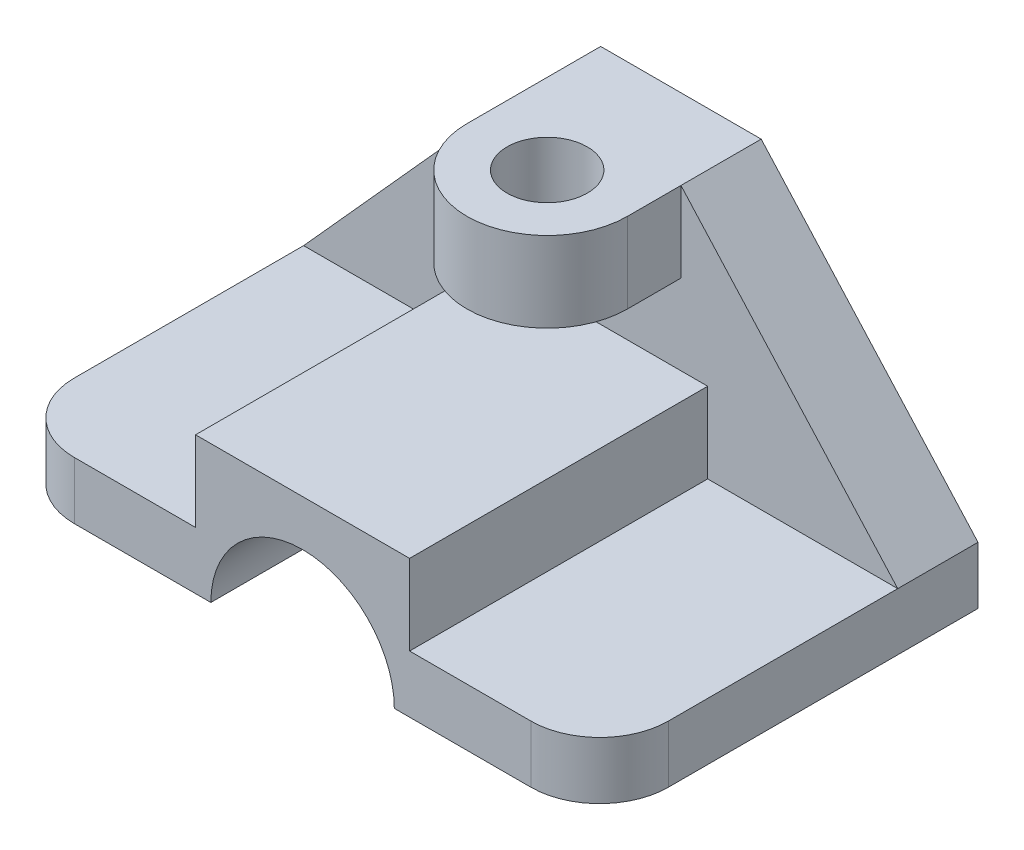
ISO-10303-21;
HEADER;
FILE_DESCRIPTION(('STEP AP214'),'2;1');
FILE_NAME('part.step','',(''),(''),'','','');
FILE_SCHEMA(('AUTOMOTIVE_DESIGN { 1 0 10303 214 1 1 1 1 }'));
ENDSEC;
DATA;
#1=APPLICATION_CONTEXT('core data for automotive mechanical design processes');
#2=APPLICATION_PROTOCOL_DEFINITION('international standard','automotive_design',2000,#1);
#3=PRODUCT_CONTEXT('',#1,'mechanical');
#4=PRODUCT('Part','Part','',(#3));
#5=PRODUCT_RELATED_PRODUCT_CATEGORY('part','',(#4));
#6=PRODUCT_DEFINITION_FORMATION('','',#4);
#7=PRODUCT_DEFINITION_CONTEXT('part definition',#1,'design');
#8=PRODUCT_DEFINITION('design','',#6,#7);
#9=PRODUCT_DEFINITION_SHAPE('','',#8);
#10=(LENGTH_UNIT() NAMED_UNIT(*) SI_UNIT(.MILLI.,.METRE.));
#11=(NAMED_UNIT(*) PLANE_ANGLE_UNIT() SI_UNIT($,.RADIAN.));
#12=(NAMED_UNIT(*) SI_UNIT($,.STERADIAN.) SOLID_ANGLE_UNIT());
#13=UNCERTAINTY_MEASURE_WITH_UNIT(LENGTH_MEASURE(1.E-05),#10,'distance_accuracy_value','');
#14=(GEOMETRIC_REPRESENTATION_CONTEXT(3) GLOBAL_UNCERTAINTY_ASSIGNED_CONTEXT((#13)) GLOBAL_UNIT_ASSIGNED_CONTEXT((#10,
#11,#12)) REPRESENTATION_CONTEXT('',''));
#15=CARTESIAN_POINT('',(0.,0.,0.));
#16=DIRECTION('',(0.,0.,1.));
#17=DIRECTION('',(1.,0.,0.));
#18=AXIS2_PLACEMENT_3D('',#15,#16,#17);
#19=CARTESIAN_POINT('',(-77.7254547907637,-57.,-14.));
#20=DIRECTION('',(0.,-1.,0.));
#21=DIRECTION('',(0.,0.,-1.));
#22=AXIS2_PLACEMENT_3D('',#19,#20,#21);
#23=PLANE('',#22);
#24=DIRECTION('',(0.,0.,1.));
#25=VECTOR('',#24,1.);
#26=CARTESIAN_POINT('',(24.,-57.,-35.001));
#27=LINE('',#26,#25);
#28=CARTESIAN_POINT('',(24.,-57.,-35.));
#29=VERTEX_POINT('',#28);
#30=CARTESIAN_POINT('',(24.,-57.,64.));
#31=VERTEX_POINT('',#30);
#32=EDGE_CURVE('E53',#29,#31,#27,.T.);
#33=ORIENTED_EDGE('',*,*,#32,.F.);
#34=DIRECTION('',(-1.,0.,0.));
#35=VECTOR('',#34,1.);
#36=CARTESIAN_POINT('',(-77.7254547907637,-57.,-35.));
#37=LINE('',#36,#35);
#38=CARTESIAN_POINT('',(77.7254547907637,-57.,-35.));
#39=VERTEX_POINT('',#38);
#40=EDGE_CURVE('E178',#39,#29,#37,.T.);
#41=ORIENTED_EDGE('',*,*,#40,.F.);
#42=DIRECTION('',(0.,0.,-1.));
#43=VECTOR('',#42,1.);
#44=CARTESIAN_POINT('',(77.7254547907637,-57.,-14.));
#45=LINE('',#44,#43);
#46=CARTESIAN_POINT('',(77.7254547907637,-57.,46.));
#47=VERTEX_POINT('',#46);
#48=EDGE_CURVE('E205',#47,#39,#45,.T.);
#49=ORIENTED_EDGE('',*,*,#48,.F.);
#50=CARTESIAN_POINT('',(59.7254547907637,-57.,46.));
#51=DIRECTION('',(0.,-1.,0.));
#52=DIRECTION('',(0.,0.,-1.));
#53=AXIS2_PLACEMENT_3D('',#50,#51,#52);
#54=CIRCLE('',#53,18.);
#55=CARTESIAN_POINT('',(59.7254547907637,-57.,64.));
#56=VERTEX_POINT('',#55);
#57=EDGE_CURVE('E258',#47,#56,#54,.T.);
#58=ORIENTED_EDGE('',*,*,#57,.T.);
#59=DIRECTION('',(1.,0.,0.));
#60=VECTOR('',#59,1.);
#61=CARTESIAN_POINT('',(-77.7254547907637,-57.,64.));
#62=LINE('',#61,#60);
#63=EDGE_CURVE('E263',#31,#56,#62,.T.);
#64=ORIENTED_EDGE('',*,*,#63,.F.);
#65=EDGE_LOOP('',(#33,#41,#49,#58,#64));
#66=FACE_BOUND('',#65,.T.);
#67=ADVANCED_FACE('F39',(#66),#23,.T.);
#68=CARTESIAN_POINT('',(0.,0.,-14.));
#69=DIRECTION('',(0.,0.,1.));
#70=DIRECTION('',(1.,0.,0.));
#71=AXIS2_PLACEMENT_3D('',#68,#69,#70);
#72=PLANE('',#71);
#73=DIRECTION('',(0.,1.,0.));
#74=VECTOR('',#73,1.);
#75=CARTESIAN_POINT('',(28.,-21.,-14.));
#76=LINE('',#75,#74);
#77=CARTESIAN_POINT('',(28.,-42.,-14.));
#78=VERTEX_POINT('',#77);
#79=CARTESIAN_POINT('',(28.,-21.,-14.));
#80=VERTEX_POINT('',#79);
#81=EDGE_CURVE('E294',#78,#80,#76,.T.);
#82=ORIENTED_EDGE('',*,*,#81,.F.);
#83=DIRECTION('',(-1.,0.,0.));
#84=VECTOR('',#83,1.);
#85=CARTESIAN_POINT('',(28.,-42.,-14.));
#86=LINE('',#85,#84);
#87=CARTESIAN_POINT('',(77.7254547907637,-42.,-14.));
#88=VERTEX_POINT('',#87);
#89=EDGE_CURVE('E295',#88,#78,#86,.T.);
#90=ORIENTED_EDGE('',*,*,#89,.F.);
#91=DIRECTION('',(0.669130606358857,-0.743144825477396,0.));
#92=VECTOR('',#91,1.);
#93=CARTESIAN_POINT('',(77.7254547907637,-42.,-14.));
#94=LINE('',#93,#92);
#95=CARTESIAN_POINT('',(21.,21.,-14.));
#96=VERTEX_POINT('',#95);
#97=EDGE_CURVE('E195',#96,#88,#94,.T.);
#98=ORIENTED_EDGE('',*,*,#97,.F.);
#99=DIRECTION('',(0.,1.,0.));
#100=VECTOR('',#99,1.);
#101=CARTESIAN_POINT('',(21.,21.,-14.));
#102=LINE('',#101,#100);
#103=CARTESIAN_POINT('',(21.,0.,-14.));
#104=VERTEX_POINT('',#103);
#105=EDGE_CURVE('E208',#104,#96,#102,.T.);
#106=ORIENTED_EDGE('',*,*,#105,.F.);
#107=DIRECTION('',(1.,0.,0.));
#108=VECTOR('',#107,1.);
#109=CARTESIAN_POINT('',(0.,0.,-14.));
#110=LINE('',#109,#108);
#111=CARTESIAN_POINT('',(-21.,0.,-14.));
#112=VERTEX_POINT('',#111);
#113=EDGE_CURVE('E196',#112,#104,#110,.T.);
#114=ORIENTED_EDGE('',*,*,#113,.F.);
#115=DIRECTION('',(0.,-1.,0.));
#116=VECTOR('',#115,1.);
#117=CARTESIAN_POINT('',(-21.,21.,-14.));
#118=LINE('',#117,#116);
#119=CARTESIAN_POINT('',(-21.,21.,-14.));
#120=VERTEX_POINT('',#119);
#121=EDGE_CURVE('E245',#120,#112,#118,.T.);
#122=ORIENTED_EDGE('',*,*,#121,.F.);
#123=DIRECTION('',(0.669130606358857,0.743144825477396,0.));
#124=VECTOR('',#123,1.);
#125=CARTESIAN_POINT('',(-21.,21.,-14.));
#126=LINE('',#125,#124);
#127=CARTESIAN_POINT('',(-77.7254547907637,-42.,-14.));
#128=VERTEX_POINT('',#127);
#129=EDGE_CURVE('E206',#128,#120,#126,.T.);
#130=ORIENTED_EDGE('',*,*,#129,.F.);
#131=DIRECTION('',(-1.,0.,0.));
#132=VECTOR('',#131,1.);
#133=CARTESIAN_POINT('',(-77.7254547907637,-42.,-14.));
#134=LINE('',#133,#132);
#135=CARTESIAN_POINT('',(-28.,-42.,-14.));
#136=VERTEX_POINT('',#135);
#137=EDGE_CURVE('E297',#136,#128,#134,.T.);
#138=ORIENTED_EDGE('',*,*,#137,.F.);
#139=DIRECTION('',(0.,-1.,0.));
#140=VECTOR('',#139,1.);
#141=CARTESIAN_POINT('',(-28.,-42.,-14.));
#142=LINE('',#141,#140);
#143=CARTESIAN_POINT('',(-28.,-21.,-14.));
#144=VERTEX_POINT('',#143);
#145=EDGE_CURVE('E296',#144,#136,#142,.T.);
#146=ORIENTED_EDGE('',*,*,#145,.F.);
#147=DIRECTION('',(-1.,0.,0.));
#148=VECTOR('',#147,1.);
#149=CARTESIAN_POINT('',(-28.,-21.,-14.));
#150=LINE('',#149,#148);
#151=EDGE_CURVE('E298',#80,#144,#150,.T.);
#152=ORIENTED_EDGE('',*,*,#151,.F.);
#153=EDGE_LOOP('',(#82,#90,#98,#106,#114,#122,#130,#138,#146,#152));
#154=FACE_BOUND('',#153,.T.);
#155=ADVANCED_FACE('F333',(#154),#72,.T.);
#156=CARTESIAN_POINT('',(0.,21.,0.));
#157=DIRECTION('',(0.,1.,0.));
#158=DIRECTION('',(0.,0.,1.));
#159=AXIS2_PLACEMENT_3D('',#156,#157,#158);
#160=PLANE('',#159);
#161=DIRECTION('',(0.,0.,-1.));
#162=VECTOR('',#161,1.);
#163=CARTESIAN_POINT('',(21.,21.,-35.));
#164=LINE('',#163,#162);
#165=CARTESIAN_POINT('',(21.,21.,0.));
#166=VERTEX_POINT('',#165);
#167=EDGE_CURVE('E219',#166,#96,#164,.T.);
#168=ORIENTED_EDGE('',*,*,#167,.T.);
#169=DIRECTION('',(0.,0.,-1.));
#170=VECTOR('',#169,1.);
#171=CARTESIAN_POINT('',(21.,21.,-14.));
#172=LINE('',#171,#170);
#173=CARTESIAN_POINT('',(21.,21.,-35.));
#174=VERTEX_POINT('',#173);
#175=EDGE_CURVE('E198',#96,#174,#172,.T.);
#176=ORIENTED_EDGE('',*,*,#175,.T.);
#177=DIRECTION('',(-1.,0.,0.));
#178=VECTOR('',#177,1.);
#179=CARTESIAN_POINT('',(-21.,21.,-35.));
#180=LINE('',#179,#178);
#181=CARTESIAN_POINT('',(-21.,21.,-35.));
#182=VERTEX_POINT('',#181);
#183=EDGE_CURVE('E221',#174,#182,#180,.T.);
#184=ORIENTED_EDGE('',*,*,#183,.T.);
#185=DIRECTION('',(0.,0.,1.));
#186=VECTOR('',#185,1.);
#187=CARTESIAN_POINT('',(-21.,21.,0.));
#188=LINE('',#187,#186);
#189=EDGE_CURVE('E230',#182,#120,#188,.T.);
#190=ORIENTED_EDGE('',*,*,#189,.T.);
#191=CARTESIAN_POINT('',(-21.,21.,0.));
#192=VERTEX_POINT('',#191);
#193=EDGE_CURVE('E228',#120,#192,#188,.T.);
#194=ORIENTED_EDGE('',*,*,#193,.T.);
#195=CARTESIAN_POINT('',(0.,21.,0.));
#196=DIRECTION('',(0.,1.,0.));
#197=DIRECTION('',(0.,0.,1.));
#198=AXIS2_PLACEMENT_3D('',#195,#196,#197);
#199=CIRCLE('',#198,21.);
#200=EDGE_CURVE('E220',#192,#166,#199,.T.);
#201=ORIENTED_EDGE('',*,*,#200,.T.);
#202=EDGE_LOOP('',(#168,#176,#184,#190,#194,#201));
#203=FACE_BOUND('',#202,.T.);
#204=CARTESIAN_POINT('',(0.,21.,0.));
#205=DIRECTION('',(0.,1.,0.));
#206=DIRECTION('',(0.,0.,1.));
#207=AXIS2_PLACEMENT_3D('',#204,#205,#206);
#208=CIRCLE('',#207,10.5);
#209=CARTESIAN_POINT('',(0.,21.,-10.5));
#210=VERTEX_POINT('',#209);
#211=EDGE_CURVE('E211',#210,#210,#208,.T.);
#212=ORIENTED_EDGE('',*,*,#211,.F.);
#213=EDGE_LOOP('',(#212));
#214=FACE_BOUND('',#213,.T.);
#215=ADVANCED_FACE('F368',(#203,#214),#160,.T.);
#216=CARTESIAN_POINT('',(0.,0.,0.));
#217=DIRECTION('',(0.,1.,0.));
#218=DIRECTION('',(0.,0.,1.));
#219=AXIS2_PLACEMENT_3D('',#216,#217,#218);
#220=PLANE('',#219);
#221=DIRECTION('',(0.,0.,1.));
#222=VECTOR('',#221,1.);
#223=CARTESIAN_POINT('',(-21.,0.,0.));
#224=LINE('',#223,#222);
#225=CARTESIAN_POINT('',(-21.,0.,0.));
#226=VERTEX_POINT('',#225);
#227=EDGE_CURVE('E222',#112,#226,#224,.T.);
#228=ORIENTED_EDGE('',*,*,#227,.F.);
#229=ORIENTED_EDGE('',*,*,#113,.T.);
#230=DIRECTION('',(0.,0.,-1.));
#231=VECTOR('',#230,1.);
#232=CARTESIAN_POINT('',(21.,0.,-35.));
#233=LINE('',#232,#231);
#234=CARTESIAN_POINT('',(21.,0.,0.));
#235=VERTEX_POINT('',#234);
#236=EDGE_CURVE('E234',#235,#104,#233,.T.);
#237=ORIENTED_EDGE('',*,*,#236,.F.);
#238=CARTESIAN_POINT('',(0.,0.,0.));
#239=DIRECTION('',(0.,1.,0.));
#240=DIRECTION('',(0.,0.,1.));
#241=AXIS2_PLACEMENT_3D('',#238,#239,#240);
#242=CIRCLE('',#241,21.);
#243=EDGE_CURVE('E212',#226,#235,#242,.T.);
#244=ORIENTED_EDGE('',*,*,#243,.F.);
#245=EDGE_LOOP('',(#228,#229,#237,#244));
#246=FACE_BOUND('',#245,.T.);
#247=CARTESIAN_POINT('',(0.,0.,0.));
#248=DIRECTION('',(0.,1.,0.));
#249=DIRECTION('',(0.,0.,1.));
#250=AXIS2_PLACEMENT_3D('',#247,#248,#249);
#251=CIRCLE('',#250,10.5);
#252=CARTESIAN_POINT('',(0.,0.,-10.5));
#253=VERTEX_POINT('',#252);
#254=EDGE_CURVE('E209',#253,#253,#251,.T.);
#255=ORIENTED_EDGE('',*,*,#254,.T.);
#256=EDGE_LOOP('',(#255));
#257=FACE_BOUND('',#256,.T.);
#258=ADVANCED_FACE('F374',(#246,#257),#220,.F.);
#259=CARTESIAN_POINT('',(0.,21.,0.));
#260=DIRECTION('',(0.,-1.,0.));
#261=DIRECTION('',(0.,0.,-1.));
#262=AXIS2_PLACEMENT_3D('',#259,#260,#261);
#263=CYLINDRICAL_SURFACE('',#262,21.);
#264=ORIENTED_EDGE('',*,*,#243,.T.);
#265=DIRECTION('',(0.,-1.,0.));
#266=VECTOR('',#265,1.);
#267=CARTESIAN_POINT('',(21.,21.,0.));
#268=LINE('',#267,#266);
#269=EDGE_CURVE('E239',#166,#235,#268,.T.);
#270=ORIENTED_EDGE('',*,*,#269,.F.);
#271=ORIENTED_EDGE('',*,*,#200,.F.);
#272=DIRECTION('',(0.,-1.,0.));
#273=VECTOR('',#272,1.);
#274=CARTESIAN_POINT('',(-21.,21.,0.));
#275=LINE('',#274,#273);
#276=EDGE_CURVE('E227',#192,#226,#275,.T.);
#277=ORIENTED_EDGE('',*,*,#276,.T.);
#278=EDGE_LOOP('',(#264,#270,#271,#277));
#279=FACE_BOUND('',#278,.T.);
#280=ADVANCED_FACE('F377',(#279),#263,.T.);
#281=CARTESIAN_POINT('',(21.,21.,-35.));
#282=DIRECTION('',(-1.,0.,0.));
#283=DIRECTION('',(0.,0.,1.));
#284=AXIS2_PLACEMENT_3D('',#281,#282,#283);
#285=PLANE('',#284);
#286=ORIENTED_EDGE('',*,*,#236,.T.);
#287=ORIENTED_EDGE('',*,*,#105,.T.);
#288=ORIENTED_EDGE('',*,*,#167,.F.);
#289=ORIENTED_EDGE('',*,*,#269,.T.);
#290=EDGE_LOOP('',(#286,#287,#288,#289));
#291=FACE_BOUND('',#290,.T.);
#292=ADVANCED_FACE('F385',(#291),#285,.F.);
#293=CARTESIAN_POINT('',(-21.,21.,-35.));
#294=DIRECTION('',(0.,0.,1.));
#295=DIRECTION('',(1.,0.,0.));
#296=AXIS2_PLACEMENT_3D('',#293,#294,#295);
#297=PLANE('',#296);
#298=ORIENTED_EDGE('',*,*,#40,.T.);
#299=CARTESIAN_POINT('',(0.,-57.,-35.));
#300=DIRECTION('',(0.,0.,1.));
#301=DIRECTION('',(1.,0.,0.));
#302=AXIS2_PLACEMENT_3D('',#299,#300,#301);
#303=CIRCLE('',#302,24.);
#304=CARTESIAN_POINT('',(-24.,-57.,-35.));
#305=VERTEX_POINT('',#304);
#306=EDGE_CURVE('E163',#305,#29,#303,.F.);
#307=ORIENTED_EDGE('',*,*,#306,.F.);
#308=CARTESIAN_POINT('',(-77.7254547907637,-57.,-35.));
#309=VERTEX_POINT('',#308);
#310=EDGE_CURVE('E172',#305,#309,#37,.T.);
#311=ORIENTED_EDGE('',*,*,#310,.T.);
#312=DIRECTION('',(0.,1.,0.));
#313=VECTOR('',#312,1.);
#314=CARTESIAN_POINT('',(-77.7254547907637,-42.,-35.));
#315=LINE('',#314,#313);
#316=CARTESIAN_POINT('',(-77.7254547907637,-42.,-35.));
#317=VERTEX_POINT('',#316);
#318=EDGE_CURVE('E188',#309,#317,#315,.T.);
#319=ORIENTED_EDGE('',*,*,#318,.T.);
#320=DIRECTION('',(0.669130606358857,0.743144825477396,0.));
#321=VECTOR('',#320,1.);
#322=CARTESIAN_POINT('',(-21.,21.,-35.));
#323=LINE('',#322,#321);
#324=EDGE_CURVE('E192',#317,#182,#323,.T.);
#325=ORIENTED_EDGE('',*,*,#324,.T.);
#326=ORIENTED_EDGE('',*,*,#183,.F.);
#327=DIRECTION('',(0.669130606358857,-0.743144825477396,0.));
#328=VECTOR('',#327,1.);
#329=CARTESIAN_POINT('',(77.7254547907637,-42.,-35.));
#330=LINE('',#329,#328);
#331=CARTESIAN_POINT('',(77.7254547907637,-42.,-35.));
#332=VERTEX_POINT('',#331);
#333=EDGE_CURVE('E190',#174,#332,#330,.T.);
#334=ORIENTED_EDGE('',*,*,#333,.T.);
#335=DIRECTION('',(0.,-1.,0.));
#336=VECTOR('',#335,1.);
#337=CARTESIAN_POINT('',(77.7254547907637,-57.,-35.));
#338=LINE('',#337,#336);
#339=EDGE_CURVE('E184',#332,#39,#338,.T.);
#340=ORIENTED_EDGE('',*,*,#339,.T.);
#341=EDGE_LOOP('',(#298,#307,#311,#319,#325,#326,#334,#340));
#342=FACE_BOUND('',#341,.T.);
#343=ADVANCED_FACE('F171',(#342),#297,.F.);
#344=CARTESIAN_POINT('',(-21.,21.,0.));
#345=DIRECTION('',(1.,0.,0.));
#346=DIRECTION('',(0.,0.,-1.));
#347=AXIS2_PLACEMENT_3D('',#344,#345,#346);
#348=PLANE('',#347);
#349=ORIENTED_EDGE('',*,*,#193,.F.);
#350=ORIENTED_EDGE('',*,*,#121,.T.);
#351=ORIENTED_EDGE('',*,*,#227,.T.);
#352=ORIENTED_EDGE('',*,*,#276,.F.);
#353=EDGE_LOOP('',(#349,#350,#351,#352));
#354=FACE_BOUND('',#353,.T.);
#355=ADVANCED_FACE('F375',(#354),#348,.F.);
#356=CARTESIAN_POINT('',(0.,21.,0.));
#357=DIRECTION('',(0.,-1.,0.));
#358=DIRECTION('',(0.,0.,-1.));
#359=AXIS2_PLACEMENT_3D('',#356,#357,#358);
#360=CYLINDRICAL_SURFACE('',#359,10.5);
#361=CARTESIAN_POINT('',(0.,21.,-10.5));
#362=CARTESIAN_POINT('',(0.,20.78125,-10.5));
#363=CARTESIAN_POINT('',(0.,20.5625,-10.5));
#364=CARTESIAN_POINT('',(0.,20.125,-10.5));
#365=CARTESIAN_POINT('',(0.,19.90625,-10.5));
#366=CARTESIAN_POINT('',(0.,19.46875,-10.5));
#367=CARTESIAN_POINT('',(0.,19.25,-10.5));
#368=CARTESIAN_POINT('',(0.,18.8125,-10.5));
#369=CARTESIAN_POINT('',(0.,18.59375,-10.5));
#370=CARTESIAN_POINT('',(0.,18.15625,-10.5));
#371=CARTESIAN_POINT('',(0.,17.9375,-10.5));
#372=CARTESIAN_POINT('',(0.,17.5,-10.5));
#373=CARTESIAN_POINT('',(0.,17.28125,-10.5));
#374=CARTESIAN_POINT('',(0.,16.84375,-10.5));
#375=CARTESIAN_POINT('',(0.,16.625,-10.5));
#376=CARTESIAN_POINT('',(0.,16.1875,-10.5));
#377=CARTESIAN_POINT('',(0.,15.96875,-10.5));
#378=CARTESIAN_POINT('',(0.,15.53125,-10.5));
#379=CARTESIAN_POINT('',(0.,15.3125,-10.5));
#380=CARTESIAN_POINT('',(0.,14.875,-10.5));
#381=CARTESIAN_POINT('',(0.,14.65625,-10.5));
#382=CARTESIAN_POINT('',(0.,14.21875,-10.5));
#383=CARTESIAN_POINT('',(0.,14.,-10.5));
#384=CARTESIAN_POINT('',(0.,13.5625,-10.5));
#385=CARTESIAN_POINT('',(0.,13.34375,-10.5));
#386=CARTESIAN_POINT('',(0.,12.90625,-10.5));
#387=CARTESIAN_POINT('',(0.,12.6875,-10.5));
#388=CARTESIAN_POINT('',(0.,12.25,-10.5));
#389=CARTESIAN_POINT('',(0.,12.03125,-10.5));
#390=CARTESIAN_POINT('',(0.,11.59375,-10.5));
#391=CARTESIAN_POINT('',(0.,11.375,-10.5));
#392=CARTESIAN_POINT('',(0.,10.9375,-10.5));
#393=CARTESIAN_POINT('',(0.,10.71875,-10.5));
#394=CARTESIAN_POINT('',(0.,10.28125,-10.5));
#395=CARTESIAN_POINT('',(0.,10.0625,-10.5));
#396=CARTESIAN_POINT('',(0.,9.625,-10.5));
#397=CARTESIAN_POINT('',(0.,9.40625,-10.5));
#398=CARTESIAN_POINT('',(0.,8.96875,-10.5));
#399=CARTESIAN_POINT('',(0.,8.75,-10.5));
#400=CARTESIAN_POINT('',(0.,8.3125,-10.5));
#401=CARTESIAN_POINT('',(0.,8.09375,-10.5));
#402=CARTESIAN_POINT('',(0.,7.65625,-10.5));
#403=CARTESIAN_POINT('',(0.,7.4375,-10.5));
#404=CARTESIAN_POINT('',(0.,7.,-10.5));
#405=CARTESIAN_POINT('',(0.,6.78125,-10.5));
#406=CARTESIAN_POINT('',(0.,6.34375,-10.5));
#407=CARTESIAN_POINT('',(0.,6.125,-10.5));
#408=CARTESIAN_POINT('',(0.,5.6875,-10.5));
#409=CARTESIAN_POINT('',(0.,5.46875,-10.5));
#410=CARTESIAN_POINT('',(0.,5.03125,-10.5));
#411=CARTESIAN_POINT('',(0.,4.8125,-10.5));
#412=CARTESIAN_POINT('',(0.,4.375,-10.5));
#413=CARTESIAN_POINT('',(0.,4.15625,-10.5));
#414=CARTESIAN_POINT('',(0.,3.71875,-10.5));
#415=CARTESIAN_POINT('',(0.,3.5,-10.5));
#416=CARTESIAN_POINT('',(0.,3.0625,-10.5));
#417=CARTESIAN_POINT('',(0.,2.84375,-10.5));
#418=CARTESIAN_POINT('',(0.,2.40625,-10.5));
#419=CARTESIAN_POINT('',(0.,2.1875,-10.5));
#420=CARTESIAN_POINT('',(0.,1.75,-10.5));
#421=CARTESIAN_POINT('',(0.,1.53125,-10.5));
#422=CARTESIAN_POINT('',(0.,1.09375,-10.5));
#423=CARTESIAN_POINT('',(0.,0.875000000000001,-10.5));
#424=CARTESIAN_POINT('',(0.,0.4375,-10.5));
#425=CARTESIAN_POINT('',(0.,0.21875,-10.5));
#426=CARTESIAN_POINT('',(0.,0.,-10.5));
#427=B_SPLINE_CURVE_WITH_KNOTS('',3,(#361,#362,#363,#364,#365,#366,#367,#368,#369,#370,#371,
#372,#373,#374,#375,#376,#377,#378,#379,#380,#381,#382,#383,#384,#385,#386,#387,#388,#389,#390,
#391,#392,#393,#394,#395,#396,#397,#398,#399,#400,#401,#402,#403,#404,#405,#406,#407,#408,#409,
#410,#411,#412,#413,#414,#415,#416,#417,#418,#419,#420,#421,#422,#423,#424,#425,#426),
.UNSPECIFIED.,.F.,.F.,(4,2,2,2,2,2,2,2,2,2,2,2,2,2,2,2,2,2,2,2,2,2,2,2,2,2,2,2,2,2,2,2,4),(0.,
0.656250000000001,1.3125,1.96875,2.625,3.28125,3.9375,4.59375,5.25,5.90625,6.5625,7.21875,7.875,
8.53125,9.1875,9.84375,10.5,11.15625,11.8125,12.46875,13.125,13.78125,14.4375,15.09375,15.75,
16.40625,17.0625,17.71875,18.375,19.03125,19.6875,20.34375,21.),.UNSPECIFIED.);
#428=EDGE_CURVE('BSEAM522',#210,#253,#427,.T.);
#429=ORIENTED_EDGE('',*,*,#211,.T.);
#430=ORIENTED_EDGE('',*,*,#254,.F.);
#431=ORIENTED_EDGE('',*,*,#428,.T.);
#432=ORIENTED_EDGE('',*,*,#428,.F.);
#433=EDGE_LOOP('',(#429,#431,#430,#432));
#434=FACE_BOUND('',#433,.T.);
#435=ADVANCED_FACE('F522',(#434),#360,.F.);
#436=CARTESIAN_POINT('',(77.7254547907637,-42.,-14.));
#437=DIRECTION('',(0.743144825477396,0.669130606358857,0.));
#438=DIRECTION('',(-0.669130606358857,0.743144825477396,0.));
#439=AXIS2_PLACEMENT_3D('',#436,#437,#438);
#440=PLANE('',#439);
#441=ORIENTED_EDGE('',*,*,#333,.F.);
#442=ORIENTED_EDGE('',*,*,#175,.F.);
#443=ORIENTED_EDGE('',*,*,#97,.T.);
#444=DIRECTION('',(0.,0.,-1.));
#445=VECTOR('',#444,1.);
#446=CARTESIAN_POINT('',(77.7254547907637,-42.,-14.));
#447=LINE('',#446,#445);
#448=EDGE_CURVE('E204',#88,#332,#447,.T.);
#449=ORIENTED_EDGE('',*,*,#448,.T.);
#450=EDGE_LOOP('',(#441,#442,#443,#449));
#451=FACE_BOUND('',#450,.T.);
#452=ADVANCED_FACE('F324',(#451),#440,.T.);
#453=CARTESIAN_POINT('',(-21.,21.,-14.));
#454=DIRECTION('',(-0.743144825477396,0.669130606358857,0.));
#455=DIRECTION('',(-0.669130606358857,-0.743144825477396,0.));
#456=AXIS2_PLACEMENT_3D('',#453,#454,#455);
#457=PLANE('',#456);
#458=ORIENTED_EDGE('',*,*,#324,.F.);
#459=DIRECTION('',(0.,0.,-1.));
#460=VECTOR('',#459,1.);
#461=CARTESIAN_POINT('',(-77.7254547907637,-42.,-14.));
#462=LINE('',#461,#460);
#463=EDGE_CURVE('E200',#128,#317,#462,.T.);
#464=ORIENTED_EDGE('',*,*,#463,.F.);
#465=ORIENTED_EDGE('',*,*,#129,.T.);
#466=ORIENTED_EDGE('',*,*,#189,.F.);
#467=EDGE_LOOP('',(#458,#464,#465,#466));
#468=FACE_BOUND('',#467,.T.);
#469=ADVANCED_FACE('F362',(#468),#457,.T.);
#470=CARTESIAN_POINT('',(-77.7254547907637,-42.,-14.));
#471=DIRECTION('',(-1.,0.,0.));
#472=DIRECTION('',(0.,0.,1.));
#473=AXIS2_PLACEMENT_3D('',#470,#471,#472);
#474=PLANE('',#473);
#475=DIRECTION('',(0.,0.,-1.));
#476=VECTOR('',#475,1.);
#477=CARTESIAN_POINT('',(-77.7254547907637,-57.,-14.));
#478=LINE('',#477,#476);
#479=CARTESIAN_POINT('',(-77.7254547907637,-57.,46.));
#480=VERTEX_POINT('',#479);
#481=EDGE_CURVE('E185',#480,#309,#478,.T.);
#482=ORIENTED_EDGE('',*,*,#481,.F.);
#483=DIRECTION('',(0.,-1.,0.));
#484=VECTOR('',#483,1.);
#485=CARTESIAN_POINT('',(-77.7254547907637,-42.,46.));
#486=LINE('',#485,#484);
#487=CARTESIAN_POINT('',(-77.7254547907637,-42.,46.));
#488=VERTEX_POINT('',#487);
#489=EDGE_CURVE('E50',#480,#488,#486,.F.);
#490=ORIENTED_EDGE('',*,*,#489,.T.);
#491=DIRECTION('',(0.,0.,-1.));
#492=VECTOR('',#491,1.);
#493=CARTESIAN_POINT('',(-77.7254547907637,-42.,64.));
#494=LINE('',#493,#492);
#495=EDGE_CURVE('E292',#488,#128,#494,.T.);
#496=ORIENTED_EDGE('',*,*,#495,.T.);
#497=ORIENTED_EDGE('',*,*,#463,.T.);
#498=ORIENTED_EDGE('',*,*,#318,.F.);
#499=EDGE_LOOP('',(#482,#490,#496,#497,#498));
#500=FACE_BOUND('',#499,.T.);
#501=ADVANCED_FACE('F357',(#500),#474,.T.);
#502=DIRECTION('',(0.,0.,1.));
#503=VECTOR('',#502,1.);
#504=CARTESIAN_POINT('',(-24.,-57.,-35.001));
#505=LINE('',#504,#503);
#506=CARTESIAN_POINT('',(-24.,-57.,64.));
#507=VERTEX_POINT('',#506);
#508=EDGE_CURVE('E161',#305,#507,#505,.T.);
#509=ORIENTED_EDGE('',*,*,#508,.T.);
#510=CARTESIAN_POINT('',(-59.7254547907637,-57.,64.));
#511=VERTEX_POINT('',#510);
#512=EDGE_CURVE('E276',#511,#507,#62,.T.);
#513=ORIENTED_EDGE('',*,*,#512,.F.);
#514=CARTESIAN_POINT('',(-59.7254547907637,-57.,46.));
#515=DIRECTION('',(0.,-1.,0.));
#516=DIRECTION('',(0.,0.,-1.));
#517=AXIS2_PLACEMENT_3D('',#514,#515,#516);
#518=CIRCLE('',#517,18.);
#519=EDGE_CURVE('E255',#511,#480,#518,.T.);
#520=ORIENTED_EDGE('',*,*,#519,.T.);
#521=ORIENTED_EDGE('',*,*,#481,.T.);
#522=ORIENTED_EDGE('',*,*,#310,.F.);
#523=EDGE_LOOP('',(#509,#513,#520,#521,#522));
#524=FACE_BOUND('',#523,.T.);
#525=ADVANCED_FACE('F182',(#524),#23,.T.);
#526=CARTESIAN_POINT('',(77.7254547907637,-57.,-14.));
#527=DIRECTION('',(1.,0.,0.));
#528=DIRECTION('',(0.,0.,-1.));
#529=AXIS2_PLACEMENT_3D('',#526,#527,#528);
#530=PLANE('',#529);
#531=DIRECTION('',(0.,0.,-1.));
#532=VECTOR('',#531,1.);
#533=CARTESIAN_POINT('',(77.7254547907637,-42.,64.));
#534=LINE('',#533,#532);
#535=CARTESIAN_POINT('',(77.7254547907637,-42.,46.));
#536=VERTEX_POINT('',#535);
#537=EDGE_CURVE('E314',#536,#88,#534,.T.);
#538=ORIENTED_EDGE('',*,*,#537,.F.);
#539=DIRECTION('',(0.,1.,0.));
#540=VECTOR('',#539,1.);
#541=CARTESIAN_POINT('',(77.7254547907637,-57.,46.));
#542=LINE('',#541,#540);
#543=EDGE_CURVE('E252',#536,#47,#542,.F.);
#544=ORIENTED_EDGE('',*,*,#543,.T.);
#545=ORIENTED_EDGE('',*,*,#48,.T.);
#546=ORIENTED_EDGE('',*,*,#339,.F.);
#547=ORIENTED_EDGE('',*,*,#448,.F.);
#548=EDGE_LOOP('',(#538,#544,#545,#546,#547));
#549=FACE_BOUND('',#548,.T.);
#550=ADVANCED_FACE('F328',(#549),#530,.T.);
#551=CARTESIAN_POINT('',(28.,-42.,64.));
#552=DIRECTION('',(0.,-1.,0.));
#553=DIRECTION('',(0.,0.,-1.));
#554=AXIS2_PLACEMENT_3D('',#551,#552,#553);
#555=PLANE('',#554);
#556=DIRECTION('',(-1.,0.,0.));
#557=VECTOR('',#556,1.);
#558=CARTESIAN_POINT('',(28.,-42.,64.));
#559=LINE('',#558,#557);
#560=CARTESIAN_POINT('',(59.7254547907637,-42.,64.));
#561=VERTEX_POINT('',#560);
#562=CARTESIAN_POINT('',(28.,-42.,64.));
#563=VERTEX_POINT('',#562);
#564=EDGE_CURVE('E269',#561,#563,#559,.T.);
#565=ORIENTED_EDGE('',*,*,#564,.F.);
#566=CARTESIAN_POINT('',(59.7254547907637,-42.,46.));
#567=DIRECTION('',(0.,-1.,0.));
#568=DIRECTION('',(0.,0.,-1.));
#569=AXIS2_PLACEMENT_3D('',#566,#567,#568);
#570=CIRCLE('',#569,18.);
#571=EDGE_CURVE('E250',#561,#536,#570,.F.);
#572=ORIENTED_EDGE('',*,*,#571,.T.);
#573=ORIENTED_EDGE('',*,*,#537,.T.);
#574=ORIENTED_EDGE('',*,*,#89,.T.);
#575=DIRECTION('',(0.,0.,-1.));
#576=VECTOR('',#575,1.);
#577=CARTESIAN_POINT('',(28.,-42.,64.));
#578=LINE('',#577,#576);
#579=EDGE_CURVE('E277',#563,#78,#578,.T.);
#580=ORIENTED_EDGE('',*,*,#579,.F.);
#581=EDGE_LOOP('',(#565,#572,#573,#574,#580));
#582=FACE_BOUND('',#581,.T.);
#583=ADVANCED_FACE('F272',(#582),#555,.F.);
#584=CARTESIAN_POINT('',(28.,-21.,64.));
#585=DIRECTION('',(-1.,0.,0.));
#586=DIRECTION('',(0.,0.,1.));
#587=AXIS2_PLACEMENT_3D('',#584,#585,#586);
#588=PLANE('',#587);
#589=ORIENTED_EDGE('',*,*,#81,.T.);
#590=DIRECTION('',(0.,0.,-1.));
#591=VECTOR('',#590,1.);
#592=CARTESIAN_POINT('',(28.,-21.,64.));
#593=LINE('',#592,#591);
#594=CARTESIAN_POINT('',(28.,-21.,64.));
#595=VERTEX_POINT('',#594);
#596=EDGE_CURVE('E309',#595,#80,#593,.T.);
#597=ORIENTED_EDGE('',*,*,#596,.F.);
#598=DIRECTION('',(0.,1.,0.));
#599=VECTOR('',#598,1.);
#600=CARTESIAN_POINT('',(28.,-21.,64.));
#601=LINE('',#600,#599);
#602=EDGE_CURVE('E279',#563,#595,#601,.T.);
#603=ORIENTED_EDGE('',*,*,#602,.F.);
#604=ORIENTED_EDGE('',*,*,#579,.T.);
#605=EDGE_LOOP('',(#589,#597,#603,#604));
#606=FACE_BOUND('',#605,.T.);
#607=ADVANCED_FACE('F341',(#606),#588,.F.);
#608=CARTESIAN_POINT('',(-28.,-21.,64.));
#609=DIRECTION('',(0.,-1.,0.));
#610=DIRECTION('',(0.,0.,-1.));
#611=AXIS2_PLACEMENT_3D('',#608,#609,#610);
#612=PLANE('',#611);
#613=ORIENTED_EDGE('',*,*,#151,.T.);
#614=DIRECTION('',(0.,0.,-1.));
#615=VECTOR('',#614,1.);
#616=CARTESIAN_POINT('',(-28.,-21.,64.));
#617=LINE('',#616,#615);
#618=CARTESIAN_POINT('',(-28.,-21.,64.));
#619=VERTEX_POINT('',#618);
#620=EDGE_CURVE('E307',#619,#144,#617,.T.);
#621=ORIENTED_EDGE('',*,*,#620,.F.);
#622=DIRECTION('',(-1.,0.,0.));
#623=VECTOR('',#622,1.);
#624=CARTESIAN_POINT('',(-28.,-21.,64.));
#625=LINE('',#624,#623);
#626=EDGE_CURVE('E283',#595,#619,#625,.T.);
#627=ORIENTED_EDGE('',*,*,#626,.F.);
#628=ORIENTED_EDGE('',*,*,#596,.T.);
#629=EDGE_LOOP('',(#613,#621,#627,#628));
#630=FACE_BOUND('',#629,.T.);
#631=ADVANCED_FACE('F343',(#630),#612,.F.);
#632=CARTESIAN_POINT('',(-28.,-42.,64.));
#633=DIRECTION('',(1.,0.,0.));
#634=DIRECTION('',(0.,0.,-1.));
#635=AXIS2_PLACEMENT_3D('',#632,#633,#634);
#636=PLANE('',#635);
#637=ORIENTED_EDGE('',*,*,#145,.T.);
#638=DIRECTION('',(0.,0.,-1.));
#639=VECTOR('',#638,1.);
#640=CARTESIAN_POINT('',(-28.,-42.,64.));
#641=LINE('',#640,#639);
#642=CARTESIAN_POINT('',(-28.,-42.,64.));
#643=VERTEX_POINT('',#642);
#644=EDGE_CURVE('E303',#643,#136,#641,.T.);
#645=ORIENTED_EDGE('',*,*,#644,.F.);
#646=DIRECTION('',(0.,-1.,0.));
#647=VECTOR('',#646,1.);
#648=CARTESIAN_POINT('',(-28.,-42.,64.));
#649=LINE('',#648,#647);
#650=EDGE_CURVE('E286',#619,#643,#649,.T.);
#651=ORIENTED_EDGE('',*,*,#650,.F.);
#652=ORIENTED_EDGE('',*,*,#620,.T.);
#653=EDGE_LOOP('',(#637,#645,#651,#652));
#654=FACE_BOUND('',#653,.T.);
#655=ADVANCED_FACE('F353',(#654),#636,.F.);
#656=CARTESIAN_POINT('',(-77.7254547907637,-42.,64.));
#657=DIRECTION('',(0.,-1.,0.));
#658=DIRECTION('',(0.,0.,-1.));
#659=AXIS2_PLACEMENT_3D('',#656,#657,#658);
#660=PLANE('',#659);
#661=ORIENTED_EDGE('',*,*,#495,.F.);
#662=CARTESIAN_POINT('',(-59.7254547907637,-42.,46.));
#663=DIRECTION('',(0.,-1.,0.));
#664=DIRECTION('',(0.,0.,-1.));
#665=AXIS2_PLACEMENT_3D('',#662,#663,#664);
#666=CIRCLE('',#665,18.);
#667=CARTESIAN_POINT('',(-59.7254547907637,-42.,64.));
#668=VERTEX_POINT('',#667);
#669=EDGE_CURVE('E11',#488,#668,#666,.F.);
#670=ORIENTED_EDGE('',*,*,#669,.T.);
#671=DIRECTION('',(-1.,0.,0.));
#672=VECTOR('',#671,1.);
#673=CARTESIAN_POINT('',(-77.7254547907637,-42.,64.));
#674=LINE('',#673,#672);
#675=EDGE_CURVE('E289',#643,#668,#674,.T.);
#676=ORIENTED_EDGE('',*,*,#675,.F.);
#677=ORIENTED_EDGE('',*,*,#644,.T.);
#678=ORIENTED_EDGE('',*,*,#137,.T.);
#679=EDGE_LOOP('',(#661,#670,#676,#677,#678));
#680=FACE_BOUND('',#679,.T.);
#681=ADVANCED_FACE('F354',(#680),#660,.F.);
#682=CARTESIAN_POINT('',(0.,0.,64.));
#683=DIRECTION('',(0.,0.,1.));
#684=DIRECTION('',(1.,0.,0.));
#685=AXIS2_PLACEMENT_3D('',#682,#683,#684);
#686=PLANE('',#685);
#687=CARTESIAN_POINT('',(0.,-57.,64.));
#688=DIRECTION('',(0.,0.,1.));
#689=DIRECTION('',(-1.,0.,0.));
#690=AXIS2_PLACEMENT_3D('',#687,#688,#689);
#691=CIRCLE('',#690,24.);
#692=EDGE_CURVE('E164',#31,#507,#691,.T.);
#693=ORIENTED_EDGE('',*,*,#692,.F.);
#694=ORIENTED_EDGE('',*,*,#63,.T.);
#695=DIRECTION('',(0.,1.,0.));
#696=VECTOR('',#695,1.);
#697=CARTESIAN_POINT('',(59.7254547907637,0.,64.));
#698=LINE('',#697,#696);
#699=EDGE_CURVE('E247',#56,#561,#698,.T.);
#700=ORIENTED_EDGE('',*,*,#699,.T.);
#701=ORIENTED_EDGE('',*,*,#564,.T.);
#702=ORIENTED_EDGE('',*,*,#602,.T.);
#703=ORIENTED_EDGE('',*,*,#626,.T.);
#704=ORIENTED_EDGE('',*,*,#650,.T.);
#705=ORIENTED_EDGE('',*,*,#675,.T.);
#706=DIRECTION('',(0.,-1.,0.));
#707=VECTOR('',#706,1.);
#708=CARTESIAN_POINT('',(-59.7254547907637,0.,64.));
#709=LINE('',#708,#707);
#710=EDGE_CURVE('E244',#668,#511,#709,.T.);
#711=ORIENTED_EDGE('',*,*,#710,.T.);
#712=ORIENTED_EDGE('',*,*,#512,.T.);
#713=EDGE_LOOP('',(#693,#694,#700,#701,#702,#703,#704,#705,#711,#712));
#714=FACE_BOUND('',#713,.T.);
#715=ADVANCED_FACE('F267',(#714),#686,.T.);
#716=CARTESIAN_POINT('',(59.7254547907637,0.,46.));
#717=DIRECTION('',(0.,1.,0.));
#718=DIRECTION('',(0.,0.,1.));
#719=AXIS2_PLACEMENT_3D('',#716,#717,#718);
#720=CYLINDRICAL_SURFACE('',#719,18.);
#721=ORIENTED_EDGE('',*,*,#57,.F.);
#722=ORIENTED_EDGE('',*,*,#543,.F.);
#723=ORIENTED_EDGE('',*,*,#571,.F.);
#724=ORIENTED_EDGE('',*,*,#699,.F.);
#725=EDGE_LOOP('',(#721,#722,#723,#724));
#726=FACE_BOUND('',#725,.T.);
#727=ADVANCED_FACE('F266',(#726),#720,.T.);
#728=CARTESIAN_POINT('',(-59.7254547907637,0.,46.));
#729=DIRECTION('',(0.,-1.,0.));
#730=DIRECTION('',(0.,0.,-1.));
#731=AXIS2_PLACEMENT_3D('',#728,#729,#730);
#732=CYLINDRICAL_SURFACE('',#731,18.);
#733=ORIENTED_EDGE('',*,*,#669,.F.);
#734=ORIENTED_EDGE('',*,*,#489,.F.);
#735=ORIENTED_EDGE('',*,*,#519,.F.);
#736=ORIENTED_EDGE('',*,*,#710,.F.);
#737=EDGE_LOOP('',(#733,#734,#735,#736));
#738=FACE_BOUND('',#737,.T.);
#739=ADVANCED_FACE('F41',(#738),#732,.T.);
#740=CARTESIAN_POINT('',(0.,-57.,-35.001));
#741=DIRECTION('',(0.,0.,1.));
#742=DIRECTION('',(1.,0.,0.));
#743=AXIS2_PLACEMENT_3D('',#740,#741,#742);
#744=CYLINDRICAL_SURFACE('',#743,24.);
#745=ORIENTED_EDGE('',*,*,#306,.T.);
#746=ORIENTED_EDGE('',*,*,#32,.T.);
#747=ORIENTED_EDGE('',*,*,#692,.T.);
#748=ORIENTED_EDGE('',*,*,#508,.F.);
#749=EDGE_LOOP('',(#745,#746,#747,#748));
#750=FACE_BOUND('',#749,.T.);
#751=ADVANCED_FACE('F162',(#750),#744,.F.);
#752=CLOSED_SHELL('',(#67,#155,#215,#258,#280,#292,#343,#355,#435,#452,#469,#501,#525,#550,#583,
#607,#631,#655,#681,#715,#727,#739,#751));
#753=MANIFOLD_SOLID_BREP('B2',#752);
#754=ADVANCED_BREP_SHAPE_REPRESENTATION('',(#18,#753),#14);
#755=SHAPE_DEFINITION_REPRESENTATION(#9,#754);
ENDSEC;
END-ISO-10303-21;
